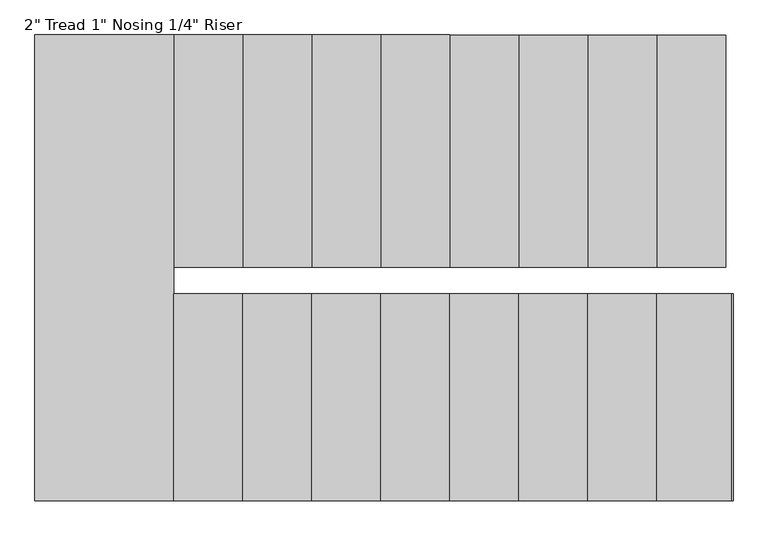
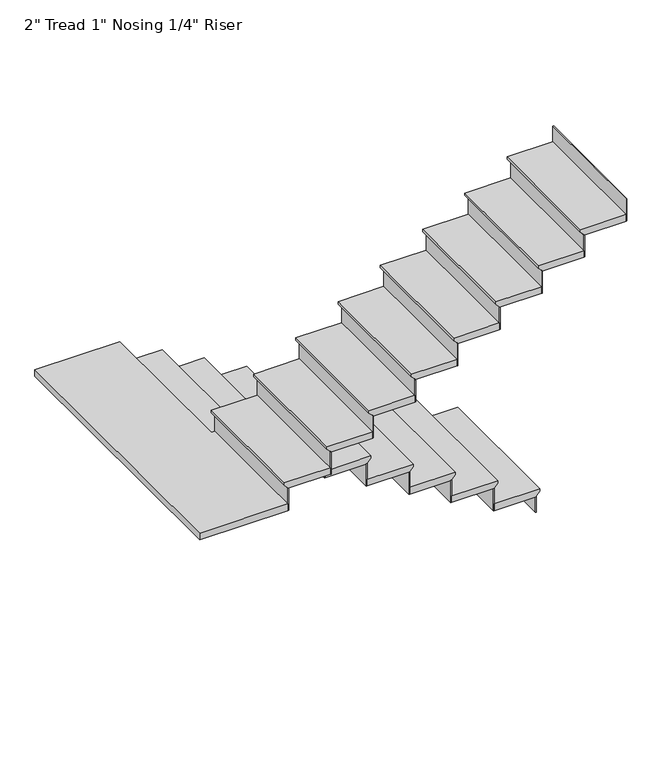
"""IFC4 building model written with IfcOpenShell, lengths in millimetres: stair flight geometry."""

from ifc_helpers import new_model, si_unit, origin, place, context, project, spatial, faceted_brep, source, transform, mapped, element, save


def stair_flight_99e02ff8(model_context):
    return source(origin(), model_context, "Body", "Brep", [
        faceted_brep([(4295.1355783, 9969.5, 12342.2833333), (4295.1355783, 9969.5, 12361.3333333), (4295.1355783, 8944.6068332, 12361.3333333), (4295.1355783, 8944.6068332, 12342.2833333), (4269.7355783, 9969.5, 12316.8833333), (4269.7355783, 8944.6068332, 12316.8833333), (3964.9355783, 9969.5, 12361.3333333), (3964.9355783, 8944.6068332, 12361.3333333), (4269.7355783, 8944.6068332, 12310.5333333), (3964.9355783, 8944.6068332, 12310.5333333), (3964.9355783, 9969.5, 12310.5333333), (4269.7355783, 9969.5, 12310.5333333)], [[[0, 1, 2, 3]], [[4, 0, 3, 5]], [[2, 1, 6, 7]], [[8, 9, 10, 11]], [[2, 7, 9, 8, 5, 3]], [[8, 11, 4, 5]], [[6, 1, 0, 4, 11, 10]], [[7, 6, 10, 9]]]),
        faceted_brep([(4269.7355783, 9969.5, 12310.5333333), (4269.7355783, 9969.5, 12192.0), (4263.3855783, 9969.5, 12192.0), (4263.3855783, 9969.5, 12310.5333333), (4269.7355783, 8944.6068332, 12310.5333333), (4263.3855783, 8944.6068332, 12310.5333333), (4263.3855783, 8944.6068332, 12192.0), (4269.7355783, 8944.6068332, 12192.0)], [[[0, 1, 2, 3]], [[4, 5, 6, 7]], [[1, 0, 4, 7]], [[2, 1, 7, 6]], [[3, 2, 6, 5]], [[0, 3, 5, 4]]]),
        faceted_brep([(3964.9355783, 9969.5, 12479.8666667), (3964.9355783, 9969.5, 12310.5333333), (3958.5855783, 9969.5, 12310.5333333), (3958.5855783, 9969.5, 12479.8666667), (3964.9355783, 8944.6068332, 12479.8666667), (3958.5855783, 8944.6068332, 12479.8666667), (3958.5855783, 8944.6068332, 12310.5333333), (3964.9355783, 8944.6068332, 12310.5333333)], [[[0, 1, 2, 3]], [[4, 5, 6, 7]], [[1, 0, 4, 7]], [[2, 1, 7, 6]], [[3, 2, 6, 5]], [[0, 3, 5, 4]]]),
        faceted_brep([(3990.3355783, 8944.6068332, 12530.6666667), (3990.3355783, 9969.5, 12530.6666667), (3660.1355783, 9969.5, 12530.6666667), (3660.1355783, 8944.6068332, 12530.6666667), (3964.9355783, 8944.6068332, 12479.8666667), (3660.1355783, 8944.6068332, 12479.8666667), (3660.1355783, 9969.5, 12479.8666667), (3964.9355783, 9969.5, 12479.8666667), (3964.9355783, 8944.6068332, 12486.2166667), (3990.3355783, 8944.6068332, 12511.6166667), (3964.9355783, 9969.5, 12486.2166667), (3990.3355783, 9969.5, 12511.6166667)], [[[0, 1, 2, 3]], [[4, 5, 6, 7]], [[0, 3, 5, 4, 8, 9]], [[4, 7, 10, 8]], [[2, 1, 11, 10, 7, 6]], [[3, 2, 6, 5]], [[11, 1, 0, 9]], [[10, 11, 9, 8]]]),
        faceted_brep([(3660.1355783, 9969.5, 12649.2), (3660.1355783, 9969.5, 12479.8666667), (3653.7855783, 9969.5, 12479.8666667), (3653.7855783, 9969.5, 12649.2), (3660.1355783, 8944.6068332, 12649.2), (3653.7855783, 8944.6068332, 12649.2), (3653.7855783, 8944.6068332, 12479.8666667), (3660.1355783, 8944.6068332, 12479.8666667)], [[[0, 1, 2, 3]], [[4, 5, 6, 7]], [[1, 0, 4, 7]], [[2, 1, 7, 6]], [[3, 2, 6, 5]], [[0, 3, 5, 4]]]),
        faceted_brep([(3685.5355783, 8944.6068332, 12700.0), (3685.5355783, 9969.5, 12700.0), (3355.3355783, 9969.5, 12700.0), (3355.3355783, 8944.6068332, 12700.0), (3660.1355783, 8944.6068332, 12649.2), (3355.3355783, 8944.6068332, 12649.2), (3355.3355783, 9969.5, 12649.2), (3660.1355783, 9969.5, 12649.2), (3660.1355783, 8944.6068332, 12655.55), (3685.5355783, 8944.6068332, 12680.95), (3660.1355783, 9969.5, 12655.55), (3685.5355783, 9969.5, 12680.95)], [[[0, 1, 2, 3]], [[4, 5, 6, 7]], [[0, 3, 5, 4, 8, 9]], [[4, 7, 10, 8]], [[2, 1, 11, 10, 7, 6]], [[3, 2, 6, 5]], [[11, 1, 0, 9]], [[10, 11, 9, 8]]]),
        faceted_brep([(3355.3355783, 9969.5, 12818.5333333), (3355.3355783, 9969.5, 12649.2), (3348.9855783, 9969.5, 12649.2), (3348.9855783, 9969.5, 12818.5333333), (3355.3355783, 8944.6068332, 12818.5333333), (3348.9855783, 8944.6068332, 12818.5333333), (3348.9855783, 8944.6068332, 12649.2), (3355.3355783, 8944.6068332, 12649.2)], [[[0, 1, 2, 3]], [[4, 5, 6, 7]], [[1, 0, 4, 7]], [[2, 1, 7, 6]], [[3, 2, 6, 5]], [[0, 3, 5, 4]]]),
        faceted_brep([(3380.7355783, 8944.6068332, 12869.3333333), (3380.7355783, 9969.5, 12869.3333333), (3050.5355783, 9969.5, 12869.3333333), (3050.5355783, 8944.6068332, 12869.3333333), (3355.3355783, 8944.6068332, 12818.5333333), (3050.5355783, 8944.6068332, 12818.5333333), (3050.5355783, 9969.5, 12818.5333333), (3355.3355783, 9969.5, 12818.5333333), (3355.3355783, 8944.6068332, 12824.8833333), (3380.7355783, 8944.6068332, 12850.2833333), (3355.3355783, 9969.5, 12824.8833333), (3380.7355783, 9969.5, 12850.2833333)], [[[0, 1, 2, 3]], [[4, 5, 6, 7]], [[0, 3, 5, 4, 8, 9]], [[4, 7, 10, 8]], [[2, 1, 11, 10, 7, 6]], [[3, 2, 6, 5]], [[11, 1, 0, 9]], [[10, 11, 9, 8]]]),
        faceted_brep([(3050.5355783, 9969.5, 12987.8666667), (3050.5355783, 9969.5, 12818.5333333), (3044.1855783, 9969.5, 12818.5333333), (3044.1855783, 9969.5, 12987.8666667), (3050.5355783, 8944.6068332, 12987.8666667), (3044.1855783, 8944.6068332, 12987.8666667), (3044.1855783, 8944.6068332, 12818.5333333), (3050.5355783, 8944.6068332, 12818.5333333)], [[[0, 1, 2, 3]], [[4, 5, 6, 7]], [[1, 0, 4, 7]], [[2, 1, 7, 6]], [[3, 2, 6, 5]], [[0, 3, 5, 4]]]),
        faceted_brep([(3075.9355783, 8944.6068332, 13038.6666667), (3075.9355783, 9969.5, 13038.6666667), (2745.7355783, 9969.5, 13038.6666667), (2745.7355783, 8944.6068332, 13038.6666667), (3050.5355783, 8944.6068332, 12987.8666667), (2745.7355783, 8944.6068332, 12987.8666667), (2745.7355783, 9969.5, 12987.8666667), (3050.5355783, 9969.5, 12987.8666667), (3050.5355783, 8944.6068332, 12994.2166667), (3075.9355783, 8944.6068332, 13019.6166667), (3050.5355783, 9969.5, 12994.2166667), (3075.9355783, 9969.5, 13019.6166667)], [[[0, 1, 2, 3]], [[4, 5, 6, 7]], [[0, 3, 5, 4, 8, 9]], [[4, 7, 10, 8]], [[2, 1, 11, 10, 7, 6]], [[3, 2, 6, 5]], [[11, 1, 0, 9]], [[10, 11, 9, 8]]]),
        faceted_brep([(2745.7355783, 9969.5, 13157.2), (2745.7355783, 9969.5, 12987.8666667), (2739.3855783, 9969.5, 12987.8666667), (2739.3855783, 9969.5, 13157.2), (2745.7355783, 8944.6068332, 13157.2), (2739.3855783, 8944.6068332, 13157.2), (2739.3855783, 8944.6068332, 12987.8666667), (2745.7355783, 8944.6068332, 12987.8666667)], [[[0, 1, 2, 3]], [[4, 5, 6, 7]], [[1, 0, 4, 7]], [[2, 1, 7, 6]], [[3, 2, 6, 5]], [[0, 3, 5, 4]]]),
        faceted_brep([(2771.1355783, 8944.6068332, 13208.0), (2771.1355783, 9969.5, 13208.0), (2440.9355783, 9969.5, 13208.0), (2440.9355783, 8944.6068332, 13208.0), (2745.7355783, 8944.6068332, 13157.2), (2440.9355783, 8944.6068332, 13157.2), (2440.9355783, 9969.5, 13157.2), (2745.7355783, 9969.5, 13157.2), (2745.7355783, 8944.6068332, 13163.55), (2771.1355783, 8944.6068332, 13188.95), (2745.7355783, 9969.5, 13163.55), (2771.1355783, 9969.5, 13188.95)], [[[0, 1, 2, 3]], [[4, 5, 6, 7]], [[0, 3, 5, 4, 8, 9]], [[4, 7, 10, 8]], [[2, 1, 11, 10, 7, 6]], [[3, 2, 6, 5]], [[11, 1, 0, 9]], [[10, 11, 9, 8]]]),
        faceted_brep([(2440.9355783, 9969.5, 13326.5333333), (2440.9355783, 9969.5, 13157.2), (2434.5855783, 9969.5, 13157.2), (2434.5855783, 9969.5, 13326.5333333), (2440.9355783, 8944.6068332, 13326.5333333), (2434.5855783, 8944.6068332, 13326.5333333), (2434.5855783, 8944.6068332, 13157.2), (2440.9355783, 8944.6068332, 13157.2)], [[[0, 1, 2, 3]], [[4, 5, 6, 7]], [[1, 0, 4, 7]], [[2, 1, 7, 6]], [[3, 2, 6, 5]], [[0, 3, 5, 4]]]),
        faceted_brep([(2466.3355783, 8944.6068332, 13377.3333333), (2466.3355783, 9969.5, 13377.3333333), (2136.1355783, 9969.5, 13377.3333333), (2136.1355783, 8944.6068332, 13377.3333333), (2440.9355783, 8944.6068332, 13326.5333333), (2136.1355783, 8944.6068332, 13326.5333333), (2136.1355783, 9969.5, 13326.5333333), (2440.9355783, 9969.5, 13326.5333333), (2440.9355783, 8944.6068332, 13332.8833333), (2466.3355783, 8944.6068332, 13358.2833333), (2440.9355783, 9969.5, 13332.8833333), (2466.3355783, 9969.5, 13358.2833333)], [[[0, 1, 2, 3]], [[4, 5, 6, 7]], [[0, 3, 5, 4, 8, 9]], [[4, 7, 10, 8]], [[2, 1, 11, 10, 7, 6]], [[3, 2, 6, 5]], [[11, 1, 0, 9]], [[10, 11, 9, 8]]]),
        faceted_brep([(2136.1355783, 9969.5, 13495.8666667), (2136.1355783, 9969.5, 13326.5333333), (2129.7855783, 9969.5, 13326.5333333), (2129.7855783, 9969.5, 13495.8666667), (2136.1355783, 8944.6068332, 13495.8666667), (2129.7855783, 8944.6068332, 13495.8666667), (2129.7855783, 8944.6068332, 13326.5333333), (2136.1355783, 8944.6068332, 13326.5333333)], [[[0, 1, 2, 3]], [[4, 5, 6, 7]], [[1, 0, 4, 7]], [[2, 1, 7, 6]], [[3, 2, 6, 5]], [[0, 3, 5, 4]]]),
        faceted_brep([(2161.5355783, 8944.6068332, 13546.6666667), (2161.5355783, 9969.5, 13546.6666667), (1831.3355783, 9969.5, 13546.6666667), (1831.3355783, 8944.6068332, 13546.6666667), (2136.1355783, 8944.6068332, 13495.8666667), (1831.3355783, 8944.6068332, 13495.8666667), (1831.3355783, 9969.5, 13495.8666667), (2136.1355783, 9969.5, 13495.8666667), (2136.1355783, 8944.6068332, 13502.2166667), (2161.5355783, 8944.6068332, 13527.6166667), (2136.1355783, 9969.5, 13502.2166667), (2161.5355783, 9969.5, 13527.6166667)], [[[0, 1, 2, 3]], [[4, 5, 6, 7]], [[0, 3, 5, 4, 8, 9]], [[4, 7, 10, 8]], [[2, 1, 11, 10, 7, 6]], [[3, 2, 6, 5]], [[11, 1, 0, 9]], [[10, 11, 9, 8]]]),
        faceted_brep([(1831.3355783, 9969.5, 13665.2), (1831.3355783, 9969.5, 13495.8666667), (1824.9855783, 9969.5, 13495.8666667), (1824.9855783, 9969.5, 13665.2), (1831.3355783, 8944.6068332, 13665.2), (1824.9855783, 8944.6068332, 13665.2), (1824.9855783, 8944.6068332, 13495.8666667), (1831.3355783, 8944.6068332, 13495.8666667)], [[[0, 1, 2, 3]], [[4, 5, 6, 7]], [[1, 0, 4, 7]], [[2, 1, 7, 6]], [[3, 2, 6, 5]], [[0, 3, 5, 4]]]),
        faceted_brep([(1882.1355783, 8826.5, 13716.0), (1856.7355783, 8826.5, 13716.0), (1856.7355783, 9969.5, 13716.0), (1244.6, 9969.5, 13716.0), (1244.6, 7912.1, 13716.0), (1882.1355783, 7912.1, 13716.0), (1856.7355783, 8826.5, 13665.2), (1882.1355783, 8826.5, 13665.2), (1882.1355783, 7912.1, 13665.2), (1244.6, 7912.1, 13665.2), (1244.6, 9969.5, 13665.2), (1831.3355783, 9969.5, 13665.2), (1831.3355783, 8944.6068332, 13665.2), (1856.7355783, 8944.6068332, 13665.2), (1856.7355783, 8944.6068332, 13696.95), (1856.7355783, 9969.5, 13696.95), (1831.3355783, 8944.6068332, 13671.55), (1831.3355783, 9969.5, 13671.55)], [[[0, 1, 2, 3, 4, 5]], [[6, 7, 8, 9, 10, 11, 12, 13]], [[1, 0, 7, 6]], [[2, 1, 6, 13, 14, 15]], [[13, 12, 16, 14]], [[12, 11, 17, 16]], [[3, 2, 15, 17, 11, 10]], [[4, 3, 10, 9]], [[5, 4, 9, 8]], [[0, 5, 8, 7]], [[17, 15, 14, 16]]]),
        faceted_brep([(1882.1355783, 7912.1, 13834.5333333), (1882.1355783, 7912.1, 13665.2), (1888.4855783, 7912.1, 13665.2), (1888.4855783, 7912.1, 13834.5333333), (1882.1355783, 8826.5, 13834.5333333), (1888.4855783, 8826.5, 13834.5333333), (1888.4855783, 8826.5, 13665.2), (1882.1355783, 8826.5, 13665.2)], [[[0, 1, 2, 3]], [[4, 5, 6, 7]], [[1, 0, 4, 7]], [[2, 1, 7, 6]], [[3, 2, 6, 5]], [[0, 3, 5, 4]]]),
        faceted_brep([(1856.7355783, 8826.5, 13885.3333333), (1856.7355783, 7912.1, 13885.3333333), (2186.9355783, 7912.1, 13885.3333333), (2186.9355783, 8826.5, 13885.3333333), (1882.1355783, 8826.5, 13834.5333333), (2186.9355783, 8826.5, 13834.5333333), (2186.9355783, 7912.1, 13834.5333333), (1882.1355783, 7912.1, 13834.5333333), (1882.1355783, 8826.5, 13840.8833333), (1856.7355783, 8826.5, 13866.2833333), (1882.1355783, 7912.1, 13840.8833333), (1856.7355783, 7912.1, 13866.2833333)], [[[0, 1, 2, 3]], [[4, 5, 6, 7]], [[0, 3, 5, 4, 8, 9]], [[4, 7, 10, 8]], [[2, 1, 11, 10, 7, 6]], [[3, 2, 6, 5]], [[11, 1, 0, 9]], [[10, 11, 9, 8]]]),
        faceted_brep([(2186.9355783, 7912.1, 14003.8666667), (2186.9355783, 7912.1, 13834.5333333), (2193.2855783, 7912.1, 13834.5333333), (2193.2855783, 7912.1, 14003.8666667), (2186.9355783, 8826.5, 14003.8666667), (2193.2855783, 8826.5, 14003.8666667), (2193.2855783, 8826.5, 13834.5333333), (2186.9355783, 8826.5, 13834.5333333)], [[[0, 1, 2, 3]], [[4, 5, 6, 7]], [[1, 0, 4, 7]], [[2, 1, 7, 6]], [[3, 2, 6, 5]], [[0, 3, 5, 4]]]),
        faceted_brep([(2161.5355783, 8826.5, 14054.6666667), (2161.5355783, 7912.1, 14054.6666667), (2491.7355783, 7912.1, 14054.6666667), (2491.7355783, 8826.5, 14054.6666667), (2186.9355783, 8826.5, 14003.8666667), (2491.7355783, 8826.5, 14003.8666667), (2491.7355783, 7912.1, 14003.8666667), (2186.9355783, 7912.1, 14003.8666667), (2186.9355783, 8826.5, 14010.2166667), (2161.5355783, 8826.5, 14035.6166667), (2186.9355783, 7912.1, 14010.2166667), (2161.5355783, 7912.1, 14035.6166667)], [[[0, 1, 2, 3]], [[4, 5, 6, 7]], [[0, 3, 5, 4, 8, 9]], [[4, 7, 10, 8]], [[2, 1, 11, 10, 7, 6]], [[3, 2, 6, 5]], [[11, 1, 0, 9]], [[10, 11, 9, 8]]]),
        faceted_brep([(2491.7355783, 7912.1, 14173.2), (2491.7355783, 7912.1, 14003.8666667), (2498.0855783, 7912.1, 14003.8666667), (2498.0855783, 7912.1, 14173.2), (2491.7355783, 8826.5, 14173.2), (2498.0855783, 8826.5, 14173.2), (2498.0855783, 8826.5, 14003.8666667), (2491.7355783, 8826.5, 14003.8666667)], [[[0, 1, 2, 3]], [[4, 5, 6, 7]], [[1, 0, 4, 7]], [[2, 1, 7, 6]], [[3, 2, 6, 5]], [[0, 3, 5, 4]]]),
        faceted_brep([(2466.3355783, 8826.5, 14224.0), (2466.3355783, 7912.1, 14224.0), (2796.5355783, 7912.1, 14224.0), (2796.5355783, 8826.5, 14224.0), (2491.7355783, 8826.5, 14173.2), (2796.5355783, 8826.5, 14173.2), (2796.5355783, 7912.1, 14173.2), (2491.7355783, 7912.1, 14173.2), (2491.7355783, 8826.5, 14179.55), (2466.3355783, 8826.5, 14204.95), (2491.7355783, 7912.1, 14179.55), (2466.3355783, 7912.1, 14204.95)], [[[0, 1, 2, 3]], [[4, 5, 6, 7]], [[0, 3, 5, 4, 8, 9]], [[4, 7, 10, 8]], [[2, 1, 11, 10, 7, 6]], [[3, 2, 6, 5]], [[11, 1, 0, 9]], [[10, 11, 9, 8]]]),
        faceted_brep([(2796.5355783, 7912.1, 14342.5333333), (2796.5355783, 7912.1, 14173.2), (2802.8855783, 7912.1, 14173.2), (2802.8855783, 7912.1, 14342.5333333), (2796.5355783, 8826.5, 14342.5333333), (2802.8855783, 8826.5, 14342.5333333), (2802.8855783, 8826.5, 14173.2), (2796.5355783, 8826.5, 14173.2)], [[[0, 1, 2, 3]], [[4, 5, 6, 7]], [[1, 0, 4, 7]], [[2, 1, 7, 6]], [[3, 2, 6, 5]], [[0, 3, 5, 4]]]),
        faceted_brep([(2771.1355783, 8826.5, 14393.3333333), (2771.1355783, 7912.1, 14393.3333333), (3101.3355783, 7912.1, 14393.3333333), (3101.3355783, 8826.5, 14393.3333333), (2796.5355783, 8826.5, 14342.5333333), (3101.3355783, 8826.5, 14342.5333333), (3101.3355783, 7912.1, 14342.5333333), (2796.5355783, 7912.1, 14342.5333333), (2796.5355783, 8826.5, 14348.8833333), (2771.1355783, 8826.5, 14374.2833333), (2796.5355783, 7912.1, 14348.8833333), (2771.1355783, 7912.1, 14374.2833333)], [[[0, 1, 2, 3]], [[4, 5, 6, 7]], [[0, 3, 5, 4, 8, 9]], [[4, 7, 10, 8]], [[2, 1, 11, 10, 7, 6]], [[3, 2, 6, 5]], [[11, 1, 0, 9]], [[10, 11, 9, 8]]]),
        faceted_brep([(3101.3355783, 7912.1, 14511.8666667), (3101.3355783, 7912.1, 14342.5333333), (3107.6855783, 7912.1, 14342.5333333), (3107.6855783, 7912.1, 14511.8666667), (3101.3355783, 8826.5, 14511.8666667), (3107.6855783, 8826.5, 14511.8666667), (3107.6855783, 8826.5, 14342.5333333), (3101.3355783, 8826.5, 14342.5333333)], [[[0, 1, 2, 3]], [[4, 5, 6, 7]], [[1, 0, 4, 7]], [[2, 1, 7, 6]], [[3, 2, 6, 5]], [[0, 3, 5, 4]]]),
        faceted_brep([(3075.9355783, 8826.5, 14562.6666667), (3075.9355783, 7912.1, 14562.6666667), (3406.1355783, 7912.1, 14562.6666667), (3406.1355783, 8826.5, 14562.6666667), (3101.3355783, 8826.5, 14511.8666667), (3406.1355783, 8826.5, 14511.8666667), (3406.1355783, 7912.1, 14511.8666667), (3101.3355783, 7912.1, 14511.8666667), (3101.3355783, 8826.5, 14518.2166667), (3075.9355783, 8826.5, 14543.6166667), (3101.3355783, 7912.1, 14518.2166667), (3075.9355783, 7912.1, 14543.6166667)], [[[0, 1, 2, 3]], [[4, 5, 6, 7]], [[0, 3, 5, 4, 8, 9]], [[4, 7, 10, 8]], [[2, 1, 11, 10, 7, 6]], [[3, 2, 6, 5]], [[11, 1, 0, 9]], [[10, 11, 9, 8]]]),
        faceted_brep([(3406.1355783, 7912.1, 14681.2), (3406.1355783, 7912.1, 14511.8666667), (3412.4855783, 7912.1, 14511.8666667), (3412.4855783, 7912.1, 14681.2), (3406.1355783, 8826.5, 14681.2), (3412.4855783, 8826.5, 14681.2), (3412.4855783, 8826.5, 14511.8666667), (3406.1355783, 8826.5, 14511.8666667)], [[[0, 1, 2, 3]], [[4, 5, 6, 7]], [[1, 0, 4, 7]], [[2, 1, 7, 6]], [[3, 2, 6, 5]], [[0, 3, 5, 4]]]),
        faceted_brep([(3380.7355783, 8826.5, 14732.0), (3380.7355783, 7912.1, 14732.0), (3710.9355783, 7912.1, 14732.0), (3710.9355783, 8826.5, 14732.0), (3406.1355783, 8826.5, 14681.2), (3710.9355783, 8826.5, 14681.2), (3710.9355783, 7912.1, 14681.2), (3406.1355783, 7912.1, 14681.2), (3406.1355783, 8826.5, 14687.55), (3380.7355783, 8826.5, 14712.95), (3406.1355783, 7912.1, 14687.55), (3380.7355783, 7912.1, 14712.95)], [[[0, 1, 2, 3]], [[4, 5, 6, 7]], [[0, 3, 5, 4, 8, 9]], [[4, 7, 10, 8]], [[2, 1, 11, 10, 7, 6]], [[3, 2, 6, 5]], [[11, 1, 0, 9]], [[10, 11, 9, 8]]]),
        faceted_brep([(3710.9355783, 7912.1, 14850.5333333), (3710.9355783, 7912.1, 14681.2), (3717.2855783, 7912.1, 14681.2), (3717.2855783, 7912.1, 14850.5333333), (3710.9355783, 8826.5, 14850.5333333), (3717.2855783, 8826.5, 14850.5333333), (3717.2855783, 8826.5, 14681.2), (3710.9355783, 8826.5, 14681.2)], [[[0, 1, 2, 3]], [[4, 5, 6, 7]], [[1, 0, 4, 7]], [[2, 1, 7, 6]], [[3, 2, 6, 5]], [[0, 3, 5, 4]]]),
        faceted_brep([(3685.5355783, 8826.5, 14901.3333333), (3685.5355783, 7912.1, 14901.3333333), (4015.7355783, 7912.1, 14901.3333333), (4015.7355783, 8826.5, 14901.3333333), (3710.9355783, 8826.5, 14850.5333333), (4015.7355783, 8826.5, 14850.5333333), (4015.7355783, 7912.1, 14850.5333333), (3710.9355783, 7912.1, 14850.5333333), (3710.9355783, 8826.5, 14856.8833333), (3685.5355783, 8826.5, 14882.2833333), (3710.9355783, 7912.1, 14856.8833333), (3685.5355783, 7912.1, 14882.2833333)], [[[0, 1, 2, 3]], [[4, 5, 6, 7]], [[0, 3, 5, 4, 8, 9]], [[4, 7, 10, 8]], [[2, 1, 11, 10, 7, 6]], [[3, 2, 6, 5]], [[11, 1, 0, 9]], [[10, 11, 9, 8]]]),
        faceted_brep([(4015.7355783, 7912.1, 15019.8666667), (4015.7355783, 7912.1, 14850.5333333), (4022.0855783, 7912.1, 14850.5333333), (4022.0855783, 7912.1, 15019.8666667), (4015.7355783, 8826.5, 15019.8666667), (4022.0855783, 8826.5, 15019.8666667), (4022.0855783, 8826.5, 14850.5333333), (4015.7355783, 8826.5, 14850.5333333)], [[[0, 1, 2, 3]], [[4, 5, 6, 7]], [[1, 0, 4, 7]], [[2, 1, 7, 6]], [[3, 2, 6, 5]], [[0, 3, 5, 4]]]),
        faceted_brep([(4320.5355783, 7912.1, 15189.2), (4320.5355783, 7912.1, 15019.8666667), (4326.8855783, 7912.1, 15019.8666667), (4326.8855783, 7912.1, 15189.2), (4320.5355783, 8826.5, 15189.2), (4326.8855783, 8826.5, 15189.2), (4326.8855783, 8826.5, 15019.8666667), (4320.5355783, 8826.5, 15019.8666667)], [[[0, 1, 2, 3]], [[4, 5, 6, 7]], [[1, 0, 4, 7]], [[2, 1, 7, 6]], [[3, 2, 6, 5]], [[0, 3, 5, 4]]]),
        faceted_brep([(3990.3355783, 8826.5, 15070.6666667), (3990.3355783, 7912.1, 15070.6666667), (4320.5355783, 7912.1, 15070.6666667), (4320.5355783, 8826.5, 15070.6666667), (4015.7355783, 8826.5, 15019.8666667), (4320.5355783, 8826.5, 15019.8666667), (4320.5355783, 7912.1, 15019.8666667), (4015.7355783, 7912.1, 15019.8666667), (4015.7355783, 8826.5, 15026.2166667), (3990.3355783, 8826.5, 15051.6166667), (4015.7355783, 7912.1, 15026.2166667), (3990.3355783, 7912.1, 15051.6166667)], [[[0, 1, 2, 3]], [[4, 5, 6, 7]], [[0, 3, 5, 4, 8, 9]], [[4, 7, 10, 8]], [[2, 1, 11, 10, 7, 6]], [[3, 2, 6, 5]], [[11, 1, 0, 9]], [[10, 11, 9, 8]]]),
    ])


if __name__ == "__main__":
    model = new_model("IFC4")
    model_context = context("Model", 3, world=origin())
    ifc_project = project(units=[si_unit("LENGTHUNIT", "METRE", prefix="MILLI")], contexts=[model_context])
    site = spatial("IfcSite", under=ifc_project)
    building = spatial("IfcBuilding", under=site)
    placement = place(None, origin())
    stair_flight_shape = stair_flight_99e02ff8(model_context)
    element("IfcStairFlight", 1, ObjectType="2\" Tread 1\" Nosing 1/4\" Riser", at=placement, inside=building, context=model_context, shape_type="MappedRepresentation", body=[
        mapped(stair_flight_shape, transform((0.0, 0.0, 0.0), x_axis=(1.0, 0.0, 0.0), y_axis=(0.0, 1.0, 0.0), z_axis=(0.0, 0.0, 1.0))),
    ])
    save(model, "model.ifc")
